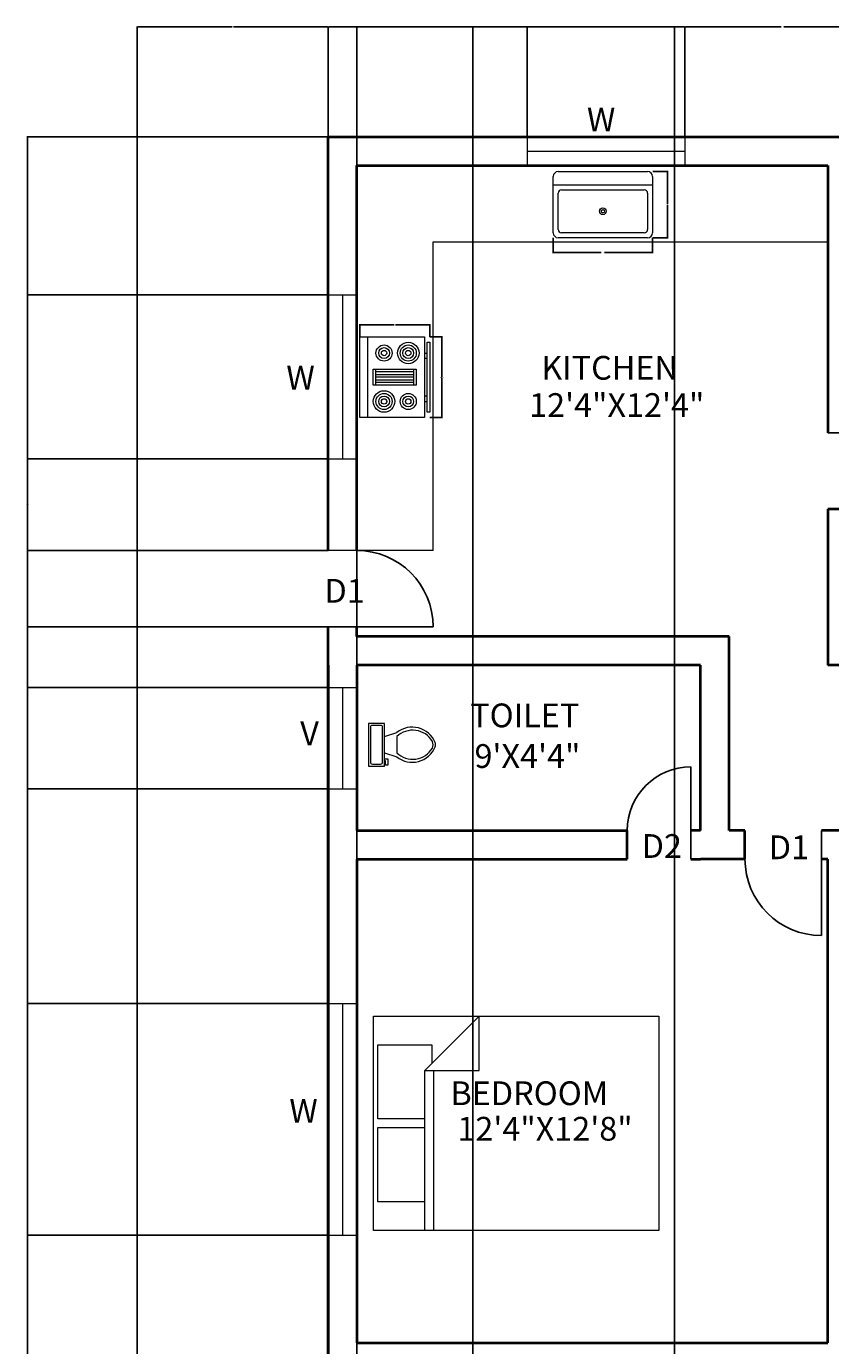
# Model space of a CAD drawing. Units: feet. Extents: x 2032 to 2763, y 1402 to 2145.
# Tile 3 of 6: x 2032 to 2285, y 1731 to 2145. Entities that reach past the tile are written whole.
import ezdxf

# ---------------------------------------------------------------- set-up
doc = ezdxf.new("R2010")
doc.units = ezdxf.units.FT
for name, color, linetype, lineweight in [('A-ANNO-DIMS', 2, 'Continuous', 18), ('A-ANNO-TEXT', 7, 'Continuous', 18), ('A-AREA-IDEN', 7, 'Continuous', 25), ('A-DOOR', 3, 'Continuous', 25), ('A-EQPM', 8, 'Continuous', 18), ('A-FLOR-CASE', 8, 'Continuous', 18), ('A-FLOR-FIXT', 8, 'Continuous', 18), ('A-FURN', 8, 'Continuous', 18), ('A-GLAZ', 4, 'Continuous', 18), ('A-WALL', 7, 'Continuous', 40), ('C-PROP', 8, 'Continuous', 25)]:
    doc.layers.add(name, color=color, linetype=linetype, lineweight=lineweight)
doc.styles.get("Standard").update_dxf_attribs({"font": 'arial.ttf'})
doc.dimstyles.get("Standard").update_dxf_attribs({"dimtxt": 0.18, "dimasz": 0.18, "dimexe": 0.18, "dimexo": 0.0625, "dimgap": 0.09, "dimtad": 0, "dimtih": 1, "dimtoh": 1, "dimdec": 4, "dimzin": 0, "dimdsep": 46, "dimtxsty": 'Standard', "dimcen": 0.09, "dimadec": 0, "dimazin": 0, "dimtfac": 1, "dimtdec": 4, "dimtofl": 0, "dimtmove": 0, "dimatfit": 3, "dimfxl": 1, "dimtolj": 1, "dimtzin": 0, "dimarcsym": 0})

# ---------------------------------------------------------------- blocks, each defined once
blk = doc.blocks.new('Sink-single - 30 in top')
blk.add_line((-15, -3.999996), (15, -3.999996))
for points in [[(-13.5, 0), (13.5, 0)], [(-15, -18.499996), (-15, -1.5)], [(15, -1.5), (15, -18.499996)], [(-13.5, -17.499996), (-13.5, -6.499996)], [(-12.5, -5.499996), (12.5, -5.499996)], [(13.5, -6.499996), (13.5, -17.499996)], [(12.5, -18.499996), (-12.5, -18.499996)], [(13.5, -19.999996), (-13.5, -19.999996)]]:
    blk.add_lwpolyline(points)
for radius in [1, 0.5]:
    blk.add_circle((0, -11.999996), radius)
for centre, radius, start, end in [((-13.5, -1.5), 1.5, 90, 180), ((13.5, -1.5), 1.5, 0, 90), ((-12.5, -6.499996), 1, 90, 180), ((12.5, -6.499996), 1, 0, 90), ((-13.5, -18.499996), 1.5, 180, 270), ((-12.5, -17.499996), 1, 180, 270), ((12.5, -17.499996), 1, 270, 0), ((13.5, -18.499996), 1.5, 270, 0)]:
    blk.add_arc(centre, radius, start, end)
blk = doc.blocks.new('Range-Oven - 30 in top')
for p, q in [((0, -3), (30, -3)), ((12, -6), (18, -6)), ((13, -20), (13, -6)), ((14, -6), (14, -20)), ((15, -20), (15, -6)), ((16, -6), (16, -20)), ((17, -20), (17, -6)), ((6, -24), (6, -25)), ((8, -25), (8, -24)), ((18, -20), (12, -20)), ((22, -25), (22, -24)), ((24, -24), (24, -25))]:
    blk.add_line(p, q)
for points in [[(0, -24), (0, 0), (30, 0), (30, -24)], [(12, -21), (12, -5), (18, -5), (18, -21)], [(2, -26), (2, -25), (28, -25), (28, -26)]]:
    blk.add_lwpolyline(points, close=True)
for centre, radius in [((6, -9), 4), ((6, -9), 3), ((6, -9), 2), ((6, -9), 1), ((24, -9), 3), ((24, -9), 2), ((24, -9), 1), ((24, -18), 4), ((6, -18), 3), ((6, -18), 2), ((6, -18), 1), ((24, -18), 3), ((24, -18), 2), ((24, -18), 1)]:
    blk.add_circle(centre, radius)
blk = doc.blocks.new('Bed - Queen')
for p, q in [((0, -80.00003), (0, 0)), ((0, 0), (59.99999, 0)), ((59.99999, 0), (59.99999, -80.00003)), ((7.99999, -1.2), (28.79998, -1.2)), ((7.99999, -14.4), (7.99999, -1.2)), ((28.79998, -1.2), (28.79998, -14.4)), ((31.19999, -1.2), (51.99999, -1.2)), ((31.19999, -14.4), (31.19999, -1.2)), ((51.99999, -1.2), (51.99999, -16.4)), ((0, -14.4), (44.8, -14.4)), ((59.99999, -29.6), (44.8, -14.4)), ((44.8, -14.4), (44.8, -29.6)), ((44.8, -16.8), (0, -16.8)), ((51.99999, -16.4), (46.79936, -16.4)), ((44.8, -29.6), (59.99999, -29.6)), ((59.99999, -80.00003), (0, -80.00003))]:
    blk.add_line(p, q)
blk = doc.blocks.new('Toilet - top')
for p, q in [((9.5, -6), (9.5, -2)), ((-10, -8.5), (-8, -8.5)), ((-10, -9.5), (-10, -8.5)), ((-7, -9.5), (-10, -9.5)), ((-8, -8.5), (-8, -8)), ((-7, -8), (-7, -9.5)), ((-4, -8), (-6, -14)), ((4, -8), (6, -14)), ((4, -14), (-4, -14))]:
    blk.add_line(p, q)
blk.add_lwpolyline([(10.5, -8), (10.5, 0), (-10.5, 0), (-10.5, -8)], close=True)
for points in [[(-9.5, -2), (-9.5, -6)], [(8.5, -1), (-8.5, -1)], [(-8.5, -7), (8.5, -7)]]:
    blk.add_lwpolyline(points)
for centre, radius, start, end in [((-8.62, -1.88), 0.884, 81.8699, 188.1301), ((-8.62, -6.12), 0.884, 171.8699, 278.1301), ((8.62, -1.88), 0.884, 351.8699, 98.1301), ((8.62, -6.12), 0.884, 261.8699, 8.1301), ((3.52, -21.58), 12.17, 141.46911, 247.97143), ((4.2, -21.82), 11.33, 136.36773, 238.94682), ((-3.52, -21.58), 12.17, 292.02843, 38.53071), ((-4.2, -21.82), 11.33, 301.05301, 43.63209), ((0, -27.88), 4, 245.73182, 294.26817), ((0, -29), 4, 254.86053, 285.13947)]:
    blk.add_arc(centre, radius, start, end)
blk = doc.blocks.new('DOOR-SWING-24')
blk.add_line((33, 0), (0, 0))
blk.add_arc((9, 0), 24, 0, 90)
blk = doc.blocks.new('DOOR-SWING-20')
blk.add_line((0, 20), (29, 20))
blk.add_arc((20, 20), 20, 180, 270)
blk = doc.blocks.new('*D27')
at = {"layer": 'A-ANNO-DIMS', "color": 0, "lineweight": -2, "transparency": 16777216}
for p, q in [((2198.05, 2078.81), (2198.05, 2074.01)), ((2229.27, 2078.81), (2229.27, 2074.01)), ((2198.23, 2074.19), (2213.13, 2074.19)), ((2229.09, 2074.19), (2214.19, 2074.19))]:
    blk.add_line(p, q, dxfattribs=at)
at = {"layer": 'A-ANNO-DIMS', "color": 0, "transparency": 16777216}
for points in [[(2198.23, 2074.22), (2198.23, 2074.16), (2198.05, 2074.19)], [(2229.09, 2074.22), (2229.09, 2074.16), (2229.27, 2074.19)]]:
    blk.add_solid(points, dxfattribs=at)
at = {"layer": 'Defpoints', "color": 0, "transparency": 16777216}
for p in [(2198.05, 2078.87), (2229.27, 2078.87), (2229.27, 2074.19)]:
    blk.add_point(p, dxfattribs=at)
at = {"layer": 'A-ANNO-DIMS', "color": 0, "transparency": 16777216, "insert": (2213.66, 2074.19), "char_height": 0.18, "attachment_point": 5}
blk.add_mtext('\\A1;SINK 31', dxfattribs=at)
blk = doc.blocks.new('*D28')
at = {"layer": 'A-ANNO-DIMS', "color": 0, "lineweight": -2, "transparency": 16777216}
for p, q in [((2229.33, 2099.68), (2234.13, 2099.68)), ((2233.95, 2099.5), (2233.95, 2089.45)), ((2233.95, 2079.05), (2233.95, 2089.09)), ((2229.33, 2078.87), (2234.13, 2078.87))]:
    blk.add_line(p, q, dxfattribs=at)
at = {"layer": 'A-ANNO-DIMS', "color": 0, "transparency": 16777216}
for points in [[(2233.92, 2099.5), (2233.98, 2099.5), (2233.95, 2099.68)], [(2233.92, 2079.05), (2233.98, 2079.05), (2233.95, 2078.87)]]:
    blk.add_solid(points, dxfattribs=at)
at = {"layer": 'Defpoints', "color": 0, "transparency": 16777216}
for p in [(2229.27, 2099.68), (2233.95, 2099.68), (2229.27, 2078.87)]:
    blk.add_point(p, dxfattribs=at)
at = {"layer": 'A-ANNO-DIMS', "color": 0, "transparency": 16777216, "insert": (2233.95, 2089.27), "char_height": 0.18, "attachment_point": 5}
blk.add_mtext('\\A1;21', dxfattribs=at)
blk = doc.blocks.new('*D29')
at = {"layer": 'A-ANNO-DIMS', "color": 0, "lineweight": -2, "transparency": 16777216}
for p, q in [((2159.3, 2047.72), (2163.22, 2047.72)), ((2163.04, 2047.54), (2163.04, 2035.22)), ((2163.04, 2022.54), (2163.04, 2034.86)), ((2159.3, 2022.36), (2163.22, 2022.36))]:
    blk.add_line(p, q, dxfattribs=at)
at = {"layer": 'A-ANNO-DIMS', "color": 0, "transparency": 16777216}
for points in [[(2163.01, 2047.54), (2163.07, 2047.54), (2163.04, 2047.72)], [(2163.01, 2022.54), (2163.07, 2022.54), (2163.04, 2022.36)]]:
    blk.add_solid(points, dxfattribs=at)
at = {"layer": 'Defpoints', "color": 0, "transparency": 16777216}
for p in [(2159.24, 2047.72), (2163.04, 2047.72), (2159.24, 2022.36)]:
    blk.add_point(p, dxfattribs=at)
at = {"layer": 'A-ANNO-DIMS', "color": 0, "transparency": 16777216, "insert": (2163.04, 2035.04), "char_height": 0.18, "attachment_point": 5}
blk.add_mtext('\\A1;RANGE 25', dxfattribs=at)
blk = doc.blocks.new('*D30')
at = {"layer": 'A-ANNO-DIMS', "color": 0, "lineweight": -2, "transparency": 16777216}
for p, q in [((2137.26, 2047.78), (2137.26, 2051.71)), ((2137.44, 2051.53), (2148.03, 2051.53)), ((2159.06, 2051.53), (2148.47, 2051.53)), ((2159.24, 2047.78), (2159.24, 2051.71))]:
    blk.add_line(p, q, dxfattribs=at)
at = {"layer": 'A-ANNO-DIMS', "color": 0, "transparency": 16777216}
for points in [[(2137.44, 2051.56), (2137.44, 2051.5), (2137.26, 2051.53)], [(2159.06, 2051.56), (2159.06, 2051.5), (2159.24, 2051.53)]]:
    blk.add_solid(points, dxfattribs=at)
at = {"layer": 'Defpoints', "color": 0, "transparency": 16777216}
for p in [(2137.26, 2051.53), (2137.26, 2047.72), (2159.24, 2047.72)]:
    blk.add_point(p, dxfattribs=at)
at = {"layer": 'A-ANNO-DIMS', "color": 0, "transparency": 16777216, "insert": (2148.25, 2051.53), "char_height": 0.18, "attachment_point": 5}
blk.add_mtext('\\A1;22', dxfattribs=at)
blk = doc.blocks.new('*D34')
at = {"layer": 'A-ANNO-DIMS', "color": 0, "lineweight": -2, "transparency": 16777216}
for p, q in [((2067.25, 2110.61), (2032.63, 2110.61)), ((2032.81, 2110.43), (2032.81, 1773.79)), ((2032.81, 1436.79), (2032.81, 1773.43)), ((2067.25, 1436.61), (2032.63, 1436.61))]:
    blk.add_line(p, q, dxfattribs=at)
at = {"layer": 'A-ANNO-DIMS', "color": 0, "transparency": 16777216}
for points in [[(2032.78, 2110.43), (2032.84, 2110.43), (2032.81, 2110.61)], [(2032.78, 1436.79), (2032.84, 1436.79), (2032.81, 1436.61)]]:
    blk.add_solid(points, dxfattribs=at)
at = {"layer": 'Defpoints', "color": 0, "transparency": 16777216}
for p in [(2032.81, 2110.61), (2067.31, 2110.61), (2067.31, 1436.61)]:
    blk.add_point(p, dxfattribs=at)
at = {"layer": 'A-ANNO-DIMS', "color": 0, "transparency": 16777216, "insert": (2032.81, 1773.61), "char_height": 0.18, "attachment_point": 5}
blk.add_mtext('\\A1;674', dxfattribs=at)
blk = doc.blocks.new('*D35')
at = {"layer": 'A-ANNO-DIMS', "color": 0, "lineweight": -2, "transparency": 16777216}
for p, q in [((2067.31, 2110.68), (2067.31, 2145.29)), ((2067.49, 2145.11), (2097.09, 2145.11)), ((2127.13, 2145.11), (2097.53, 2145.11)), ((2127.31, 2110.68), (2127.31, 2145.29))]:
    blk.add_line(p, q, dxfattribs=at)
at = {"layer": 'A-ANNO-DIMS', "color": 0, "transparency": 16777216}
for points in [[(2067.49, 2145.14), (2067.49, 2145.08), (2067.31, 2145.11)], [(2127.13, 2145.14), (2127.13, 2145.08), (2127.31, 2145.11)]]:
    blk.add_solid(points, dxfattribs=at)
at = {"layer": 'Defpoints', "color": 0, "transparency": 16777216}
for p in [(2127.31, 2145.11), (2067.31, 2110.61), (2127.31, 2110.61)]:
    blk.add_point(p, dxfattribs=at)
at = {"layer": 'A-ANNO-DIMS', "color": 0, "transparency": 16777216, "insert": (2097.31, 2145.11), "char_height": 0.18, "attachment_point": 5}
blk.add_mtext('\\A1;60', dxfattribs=at)
blk = doc.blocks.new('*D36')
at = {"layer": 'A-ANNO-DIMS', "color": 0, "lineweight": -2, "transparency": 16777216}
for p, q in [((2127.31, 2110.68), (2127.31, 2145.29)), ((2127.49, 2145.11), (2158.16, 2145.11)), ((2189.62, 2145.11), (2158.95, 2145.11)), ((2189.8, 2110.68), (2189.8, 2145.29))]:
    blk.add_line(p, q, dxfattribs=at)
at = {"layer": 'A-ANNO-DIMS', "color": 0, "transparency": 16777216}
for points in [[(2127.49, 2145.14), (2127.49, 2145.08), (2127.31, 2145.11)], [(2189.62, 2145.14), (2189.62, 2145.08), (2189.8, 2145.11)]]:
    blk.add_solid(points, dxfattribs=at)
at = {"layer": 'Defpoints', "color": 0, "transparency": 16777216}
for p in [(2189.8, 2145.11), (2127.31, 2110.61), (2189.8, 2110.61)]:
    blk.add_point(p, dxfattribs=at)
at = {"layer": 'A-ANNO-DIMS', "color": 0, "transparency": 16777216, "insert": (2158.56, 2145.11), "char_height": 0.18, "attachment_point": 5}
blk.add_mtext('\\A1;62.49', dxfattribs=at)
blk = doc.blocks.new('*D37')
at = {"layer": 'A-ANNO-DIMS', "color": 0, "lineweight": -2, "transparency": 16777216}
for p, q in [((2189.8, 2110.68), (2189.8, 2145.29)), ((2189.98, 2145.11), (2214.23, 2145.11)), ((2239.27, 2145.11), (2215.02, 2145.11)), ((2239.45, 2110.68), (2239.45, 2145.29))]:
    blk.add_line(p, q, dxfattribs=at)
at = {"layer": 'A-ANNO-DIMS', "color": 0, "transparency": 16777216}
for points in [[(2189.98, 2145.14), (2189.98, 2145.08), (2189.8, 2145.11)], [(2239.27, 2145.14), (2239.27, 2145.08), (2239.45, 2145.11)]]:
    blk.add_solid(points, dxfattribs=at)
at = {"layer": 'Defpoints', "color": 0, "transparency": 16777216}
for p in [(2239.45, 2145.11), (2189.8, 2110.61), (2239.45, 2110.61)]:
    blk.add_point(p, dxfattribs=at)
at = {"layer": 'A-ANNO-DIMS', "color": 0, "transparency": 16777216, "insert": (2214.62, 2145.11), "char_height": 0.18, "attachment_point": 5}
blk.add_mtext('\\A1;49.64', dxfattribs=at)
blk = doc.blocks.new('*D38')
at = {"layer": 'A-ANNO-DIMS', "color": 0, "lineweight": -2, "transparency": 16777216}
for p, q in [((2239.45, 2110.68), (2239.45, 2145.29)), ((2239.63, 2145.11), (2269.73, 2145.11)), ((2300.62, 2145.11), (2270.52, 2145.11)), ((2300.8, 2110.68), (2300.8, 2145.29))]:
    blk.add_line(p, q, dxfattribs=at)
at = {"layer": 'A-ANNO-DIMS', "color": 0, "transparency": 16777216}
for points in [[(2239.63, 2145.14), (2239.63, 2145.08), (2239.45, 2145.11)], [(2300.62, 2145.14), (2300.62, 2145.08), (2300.8, 2145.11)]]:
    blk.add_solid(points, dxfattribs=at)
at = {"layer": 'Defpoints', "color": 0, "transparency": 16777216}
for p in [(2300.8, 2145.11), (2239.45, 2110.61), (2300.8, 2110.61)]:
    blk.add_point(p, dxfattribs=at)
at = {"layer": 'A-ANNO-DIMS', "color": 0, "transparency": 16777216, "insert": (2270.12, 2145.11), "char_height": 0.18, "attachment_point": 5}
blk.add_mtext('\\A1;61.36', dxfattribs=at)
blk = doc.blocks.new('*D53')
at = {"layer": 'A-ANNO-DIMS', "color": 0, "lineweight": -2, "transparency": 16777216}
for p, q in [((2127.25, 1765.5), (2032.63, 1765.5)), ((2032.81, 1765.32), (2032.81, 1738.43)), ((2032.81, 1711.18), (2032.81, 1738.07)), ((2127.25, 1711), (2032.63, 1711))]:
    blk.add_line(p, q, dxfattribs=at)
at = {"layer": 'A-ANNO-DIMS', "color": 0, "transparency": 16777216}
for points in [[(2032.78, 1765.32), (2032.84, 1765.32), (2032.81, 1765.5)], [(2032.78, 1711.18), (2032.84, 1711.18), (2032.81, 1711)]]:
    blk.add_solid(points, dxfattribs=at)
at = {"layer": 'Defpoints', "color": 0, "transparency": 16777216}
for p in [(2032.81, 1765.5), (2127.31, 1765.5), (2127.31, 1711)]:
    blk.add_point(p, dxfattribs=at)
at = {"layer": 'A-ANNO-DIMS', "color": 0, "transparency": 16777216, "insert": (2032.81, 1738.25), "char_height": 0.18, "attachment_point": 5}
blk.add_mtext('\\A1;54.5', dxfattribs=at)
blk = doc.blocks.new('*D54')
at = {"layer": 'A-ANNO-DIMS', "color": 0, "lineweight": -2, "transparency": 16777216}
for p, q in [((2127.25, 1838.26), (2032.63, 1838.26)), ((2032.81, 1838.08), (2032.81, 1802.06)), ((2032.81, 1765.68), (2032.81, 1801.7)), ((2127.25, 1765.5), (2032.63, 1765.5))]:
    blk.add_line(p, q, dxfattribs=at)
at = {"layer": 'A-ANNO-DIMS', "color": 0, "transparency": 16777216}
for points in [[(2032.78, 1838.08), (2032.84, 1838.08), (2032.81, 1838.26)], [(2032.78, 1765.68), (2032.84, 1765.68), (2032.81, 1765.5)]]:
    blk.add_solid(points, dxfattribs=at)
at = {"layer": 'Defpoints', "color": 0, "transparency": 16777216}
for p in [(2032.81, 1838.26), (2127.31, 1838.26), (2127.31, 1765.5)]:
    blk.add_point(p, dxfattribs=at)
at = {"layer": 'A-ANNO-DIMS', "color": 0, "transparency": 16777216, "insert": (2032.81, 1801.88), "char_height": 0.18, "attachment_point": 5}
blk.add_mtext('\\A1;72.76', dxfattribs=at)
blk = doc.blocks.new('*D55')
at = {"layer": 'A-ANNO-DIMS', "color": 0, "lineweight": -2, "transparency": 16777216}
for p, q in [((2127.25, 1905.74), (2032.63, 1905.74)), ((2032.81, 1905.56), (2032.81, 1872.18)), ((2032.81, 1838.44), (2032.81, 1871.82)), ((2127.25, 1838.26), (2032.63, 1838.26))]:
    blk.add_line(p, q, dxfattribs=at)
at = {"layer": 'A-ANNO-DIMS', "color": 0, "transparency": 16777216}
for points in [[(2032.78, 1905.56), (2032.84, 1905.56), (2032.81, 1905.74)], [(2032.78, 1838.44), (2032.84, 1838.44), (2032.81, 1838.26)]]:
    blk.add_solid(points, dxfattribs=at)
at = {"layer": 'Defpoints', "color": 0, "transparency": 16777216}
for p in [(2032.81, 1905.74), (2127.31, 1905.74), (2127.31, 1838.26)]:
    blk.add_point(p, dxfattribs=at)
at = {"layer": 'A-ANNO-DIMS', "color": 0, "transparency": 16777216, "insert": (2032.81, 1872), "char_height": 0.18, "attachment_point": 5}
blk.add_mtext('\\A1;67.48', dxfattribs=at)
blk = doc.blocks.new('*D56')
at = {"layer": 'A-ANNO-DIMS', "color": 0, "lineweight": -2, "transparency": 16777216}
for p, q in [((2127.25, 1937.59), (2032.63, 1937.59)), ((2032.81, 1937.41), (2032.81, 1921.85)), ((2032.81, 1905.92), (2032.81, 1921.48)), ((2127.25, 1905.74), (2032.63, 1905.74))]:
    blk.add_line(p, q, dxfattribs=at)
at = {"layer": 'A-ANNO-DIMS', "color": 0, "transparency": 16777216}
for points in [[(2032.78, 1937.41), (2032.84, 1937.41), (2032.81, 1937.59)], [(2032.78, 1905.92), (2032.84, 1905.92), (2032.81, 1905.74)]]:
    blk.add_solid(points, dxfattribs=at)
at = {"layer": 'Defpoints', "color": 0, "transparency": 16777216}
for p in [(2032.81, 1937.59), (2127.31, 1937.59), (2127.31, 1905.74)]:
    blk.add_point(p, dxfattribs=at)
at = {"layer": 'A-ANNO-DIMS', "color": 0, "transparency": 16777216, "insert": (2032.81, 1921.66), "char_height": 0.18, "attachment_point": 5}
blk.add_mtext('\\A1;31.85', dxfattribs=at)
blk = doc.blocks.new('*D57')
at = {"layer": 'A-ANNO-DIMS', "color": 0, "lineweight": -2, "transparency": 16777216}
for p, q in [((2127.25, 1956.61), (2032.63, 1956.61)), ((2032.81, 1956.43), (2032.81, 1947.28)), ((2032.81, 1937.77), (2032.81, 1946.92)), ((2127.25, 1937.59), (2032.63, 1937.59))]:
    blk.add_line(p, q, dxfattribs=at)
at = {"layer": 'A-ANNO-DIMS', "color": 0, "transparency": 16777216}
for points in [[(2032.78, 1956.43), (2032.84, 1956.43), (2032.81, 1956.61)], [(2032.78, 1937.77), (2032.84, 1937.77), (2032.81, 1937.59)]]:
    blk.add_solid(points, dxfattribs=at)
at = {"layer": 'Defpoints', "color": 0, "transparency": 16777216}
for p in [(2032.81, 1956.61), (2127.31, 1956.61), (2127.31, 1937.59)]:
    blk.add_point(p, dxfattribs=at)
at = {"layer": 'A-ANNO-DIMS', "color": 0, "transparency": 16777216, "insert": (2032.81, 1947.1), "char_height": 0.18, "attachment_point": 5}
blk.add_mtext('\\A1;19.025', dxfattribs=at)
blk = doc.blocks.new('*D58')
at = {"layer": 'A-ANNO-DIMS', "color": 0, "lineweight": -2, "transparency": 16777216}
for p, q in [((2127.25, 1980.61), (2032.63, 1980.61)), ((2032.81, 1980.43), (2032.81, 1968.79)), ((2032.81, 1956.79), (2032.81, 1968.43)), ((2127.25, 1956.61), (2032.63, 1956.61))]:
    blk.add_line(p, q, dxfattribs=at)
at = {"layer": 'A-ANNO-DIMS', "color": 0, "transparency": 16777216}
for points in [[(2032.78, 1980.43), (2032.84, 1980.43), (2032.81, 1980.61)], [(2032.78, 1956.79), (2032.84, 1956.79), (2032.81, 1956.61)]]:
    blk.add_solid(points, dxfattribs=at)
at = {"layer": 'Defpoints', "color": 0, "transparency": 16777216}
for p in [(2032.81, 1980.61), (2127.31, 1980.61), (2127.31, 1956.61)]:
    blk.add_point(p, dxfattribs=at)
at = {"layer": 'A-ANNO-DIMS', "color": 0, "transparency": 16777216, "insert": (2032.81, 1968.61), "char_height": 0.18, "attachment_point": 5}
blk.add_mtext('\\A1;24', dxfattribs=at)
blk = doc.blocks.new('*D59')
at = {"layer": 'A-ANNO-DIMS', "color": 0, "lineweight": -2, "transparency": 16777216}
for p, q in [((2127.25, 2009.42), (2032.63, 2009.42)), ((2032.81, 2009.24), (2032.81, 1995.2)), ((2032.81, 1980.79), (2032.81, 1994.83)), ((2127.25, 1980.61), (2032.63, 1980.61))]:
    blk.add_line(p, q, dxfattribs=at)
at = {"layer": 'A-ANNO-DIMS', "color": 0, "transparency": 16777216}
for points in [[(2032.78, 2009.24), (2032.84, 2009.24), (2032.81, 2009.42)], [(2032.78, 1980.79), (2032.84, 1980.79), (2032.81, 1980.61)]]:
    blk.add_solid(points, dxfattribs=at)
at = {"layer": 'Defpoints', "color": 0, "transparency": 16777216}
for p in [(2032.81, 2009.42), (2127.31, 2009.42), (2127.31, 1980.61)]:
    blk.add_point(p, dxfattribs=at)
at = {"layer": 'A-ANNO-DIMS', "color": 0, "transparency": 16777216, "insert": (2032.81, 1995.02), "char_height": 0.18, "attachment_point": 5}
blk.add_mtext('\\A1;28.807', dxfattribs=at)
blk = doc.blocks.new('*D60')
at = {"layer": 'A-ANNO-DIMS', "color": 0, "lineweight": -2, "transparency": 16777216}
for p, q in [((2127.25, 2060.94), (2032.63, 2060.94)), ((2032.81, 2060.76), (2032.81, 2035.36)), ((2032.81, 2009.6), (2032.81, 2035)), ((2127.25, 2009.42), (2032.63, 2009.42))]:
    blk.add_line(p, q, dxfattribs=at)
at = {"layer": 'A-ANNO-DIMS', "color": 0, "transparency": 16777216}
for points in [[(2032.78, 2060.76), (2032.84, 2060.76), (2032.81, 2060.94)], [(2032.78, 2009.6), (2032.84, 2009.6), (2032.81, 2009.42)]]:
    blk.add_solid(points, dxfattribs=at)
at = {"layer": 'Defpoints', "color": 0, "transparency": 16777216}
for p in [(2032.81, 2060.94), (2127.31, 2060.94), (2127.31, 2009.42)]:
    blk.add_point(p, dxfattribs=at)
at = {"layer": 'A-ANNO-DIMS', "color": 0, "transparency": 16777216, "insert": (2032.81, 2035.18), "char_height": 0.18, "attachment_point": 5}
blk.add_mtext('\\A1;51.52', dxfattribs=at)
blk = doc.blocks.new('*D61')
at = {"layer": 'A-ANNO-DIMS', "color": 0, "lineweight": -2, "transparency": 16777216}
for p, q in [((2127.25, 2110.61), (2032.63, 2110.61)), ((2032.81, 2110.43), (2032.81, 2085.96)), ((2032.81, 2061.12), (2032.81, 2085.59)), ((2127.25, 2060.94), (2032.63, 2060.94))]:
    blk.add_line(p, q, dxfattribs=at)
at = {"layer": 'A-ANNO-DIMS', "color": 0, "transparency": 16777216}
for points in [[(2032.78, 2110.43), (2032.84, 2110.43), (2032.81, 2110.61)], [(2032.78, 2061.12), (2032.84, 2061.12), (2032.81, 2060.94)]]:
    blk.add_solid(points, dxfattribs=at)
at = {"layer": 'Defpoints', "color": 0, "transparency": 16777216}
for p in [(2032.81, 2110.61), (2127.31, 2110.61), (2127.31, 2060.94)]:
    blk.add_point(p, dxfattribs=at)
at = {"layer": 'A-ANNO-DIMS', "color": 0, "transparency": 16777216, "insert": (2032.81, 2085.78), "char_height": 0.18, "attachment_point": 5}
blk.add_mtext('\\A1;49.68', dxfattribs=at)
blk = doc.blocks.new('*D70')
at = {"layer": 'A-ANNO-DIMS', "color": 0, "lineweight": -2, "transparency": 16777216}
for p, q in [((2136.31, 1505.68), (2136.31, 2145.29)), ((2136.49, 2145.11), (2154.19, 2145.11)), ((2172.54, 2145.11), (2154.84, 2145.11)), ((2172.72, 1505.68), (2172.72, 2145.29))]:
    blk.add_line(p, q, dxfattribs=at)
at = {"layer": 'A-ANNO-DIMS', "color": 0, "transparency": 16777216}
for points in [[(2136.49, 2145.14), (2136.49, 2145.08), (2136.31, 2145.11)], [(2172.54, 2145.14), (2172.54, 2145.08), (2172.72, 2145.11)]]:
    blk.add_solid(points, dxfattribs=at)
at = {"layer": 'Defpoints', "color": 0, "transparency": 16777216}
for p in [(2172.72, 2145.11), (2136.31, 1505.61), (2172.72, 1505.61)]:
    blk.add_point(p, dxfattribs=at)
at = {"layer": 'A-ANNO-DIMS', "color": 0, "transparency": 16777216, "insert": (2154.51, 2145.11), "char_height": 0.18, "attachment_point": 5}
blk.add_mtext('\\A1;36.4', dxfattribs=at)
blk = doc.blocks.new('*D71')
at = {"layer": 'A-ANNO-DIMS', "color": 0, "lineweight": -2, "transparency": 16777216}
for p, q in [((2172.72, 1505.68), (2172.72, 2145.29)), ((2172.9, 2145.11), (2204.05, 2145.11)), ((2236, 2145.11), (2204.84, 2145.11)), ((2236.18, 1505.68), (2236.18, 2145.29))]:
    blk.add_line(p, q, dxfattribs=at)
at = {"layer": 'A-ANNO-DIMS', "color": 0, "transparency": 16777216}
for points in [[(2172.9, 2145.14), (2172.9, 2145.08), (2172.72, 2145.11)], [(2236, 2145.14), (2236, 2145.08), (2236.18, 2145.11)]]:
    blk.add_solid(points, dxfattribs=at)
at = {"layer": 'Defpoints', "color": 0, "transparency": 16777216}
for p in [(2236.18, 2145.11), (2172.72, 1505.61), (2236.18, 1505.61)]:
    blk.add_point(p, dxfattribs=at)
at = {"layer": 'A-ANNO-DIMS', "color": 0, "transparency": 16777216, "insert": (2204.45, 2145.11), "char_height": 0.18, "attachment_point": 5}
blk.add_mtext('\\A1;63.46', dxfattribs=at)

msp = doc.modelspace()

# ---------------------------------------------------------------- linework, layer by layer
at = {"layer": 'A-FLOR-CASE'}
for p, q in [((2160.3136, 2077.6131), (2284.3136, 2077.6131)), ((2160.3136, 1980.6131), (2160.3136, 2077.6131)), ((2160.3136, 1980.6131), (2127.3136, 1980.6131))]:
    msp.add_line(p, q, dxfattribs=at)
at = {"layer": 'A-GLAZ'}
for p, q in [((2189.8034, 2110.6131), (2189.8034, 2101.6131)), ((2239.4453, 2110.6131), (2239.4453, 2101.6131)), ((2189.8034, 2106.1131), (2239.4453, 2106.1131)), ((2127.3136, 2060.9373), (2136.3136, 2060.9373)), ((2131.8136, 2060.9373), (2131.8136, 2009.42)), ((2127.3136, 2009.42), (2136.3136, 2009.42)), ((2127.3136, 1937.5885), (2136.3136, 1937.5885)), ((2131.8136, 1937.5885), (2131.8136, 1905.7409)), ((2127.3136, 1905.7409), (2136.3136, 1905.7409)), ((2127.3136, 1838.2613), (2136.3136, 1838.2613)), ((2131.8136, 1838.2613), (2131.8136, 1765.4989)), ((2127.3136, 1765.4989), (2136.3136, 1765.4989))]:
    msp.add_line(p, q, dxfattribs=at)
at = {"layer": 'A-WALL'}
for p, q in [((2127.3136, 2110.6131), (2284.3136, 2110.6131)), ((2127.3136, 2110.6131), (2515.3136, 2110.6131)), ((2127.3136, 2110.6131), (2515.3136, 2110.6131)), ((2127.3136, 1980.6131), (2127.3136, 2110.6131)), ((2136.3136, 2101.6131), (2284.3136, 2101.6131)), ((2136.3136, 1980.6131), (2136.3136, 2101.6131)), ((2284.3136, 2101.6131), (2284.3136, 2017.6131)), ((2293.3136, 1993.6131), (2284.3136, 1993.6131)), ((2284.3136, 1993.6131), (2284.3136, 1944.6131)), ((2127.3136, 1496.6131), (2127.3136, 1956.6131)), ((2136.3136, 1953.6131), (2136.3136, 1956.6131)), ((2253.3136, 1953.6131), (2136.3136, 1953.6131)), ((2253.3136, 1892.6131), (2253.3136, 1953.6131)), ((2127.3136, 1944.6131), (2127.3136, 1496.6131)), ((2136.3136, 1944.6131), (2136.3136, 1892.6131)), ((2244.3136, 1944.6131), (2136.3136, 1944.6131)), ((2244.3136, 1892.6131), (2244.3136, 1944.6131)), ((2494.3136, 1944.6131), (2284.3136, 1944.6131)), ((2136.3136, 1892.6131), (2221.3136, 1892.6131)), ((2221.3136, 1883.6131), (2221.3136, 1892.6131)), ((2244.3136, 1892.6131), (2241.3136, 1892.6131)), ((2258.3136, 1892.6131), (2253.3136, 1892.6131)), ((2258.3136, 1883.6131), (2258.3136, 1892.6131)), ((2293.3136, 1892.6131), (2282.3136, 1892.6131)), ((2127.3136, 1883.6131), (2127.3136, 1731.6131)), ((2136.3136, 1883.6131), (2221.3136, 1883.6131)), ((2136.3136, 1883.6131), (2136.3136, 1731.6131)), ((2241.3136, 1883.6131), (2244.3136, 1883.6131)), ((2258.3136, 1883.6131), (2244.3136, 1883.6131)), ((2284.3136, 1883.6131), (2282.3136, 1883.6131)), ((2284.3136, 1731.6131), (2284.3136, 1883.6131)), ((2136.3136, 1731.6131), (2284.3136, 1731.6131))]:
    msp.add_line(p, q, dxfattribs=at)
at = {"layer": 'C-PROP'}
for p, q in [((2127.3136, 2110.6131), (2067.3136, 2110.6131)), ((2067.3136, 2110.6131), (2067.3136, 1436.6131))]:
    msp.add_line(p, q, dxfattribs=at)

# ---------------------------------------------------------------- block references
at = {"layer": 'A-DOOR', "extrusion": (0, 0, -1), "zscale": -1}
for p, rotation in [((-2284.314, 2017.6131), 180), ((-2282.3137, 1892.6127), 269.9999999999988)]:
    msp.add_blockref('DOOR-SWING-24', p, dxfattribs=dict(at, rotation=rotation))
at = {"layer": 'A-DOOR'}
msp.add_blockref('DOOR-SWING-24', (2127.314, 1956.613), dxfattribs=at)
at = {"layer": 'A-DOOR', "rotation": 270}
msp.add_blockref('DOOR-SWING-20', (2221.3136, 1912.6127), dxfattribs=at)
at = {"layer": 'A-EQPM', "xscale": 0.8453592349900645, "yscale": 0.8453592349900645, "zscale": 0.8453592349900645, "rotation": 90}
msp.add_blockref('Range-Oven - 30 in top', (2137.2578, 2022.3602), dxfattribs=at)
at = {"layer": 'A-FLOR-FIXT', "xscale": 1.04056653052336, "yscale": 1.04056653052336, "zscale": 1.04056653052336}
msp.add_blockref('Sink-single - 30 in top', (2213.6616, 2099.6798), dxfattribs=at)
at = {"layer": 'A-FLOR-FIXT', "xscale": 0.6388725113463674, "yscale": 0.6388725113463674, "zscale": 0.6388725113463674, "rotation": 90}
msp.add_blockref('Toilet - top', (2139.9337, 1919.5774), dxfattribs=at)
at = {"layer": 'A-FURN', "xscale": 1.121589901058193, "yscale": 1.121589901058193, "zscale": 1.121589901058193, "rotation": 90}
msp.add_blockref('Bed - Queen', (2141.5258, 1766.9746), dxfattribs=at)

# ---------------------------------------------------------------- texts
at = {"layer": 'A-ANNO-TEXT'}
for s, height, p in [('W', 7.4682, (2208.6287, 2112.329)), ('W', 7.4682, (2114.1497, 2031.1811)), ('D1', 7.46821, (2126.145, 1964.2018)), ('V', 7.4682, (2118.5085, 1919.4286)), ('D2', 7.46821, (2225.8265, 1884.0023)), ('D1', 7.46821, (2265.785, 1883.6085)), ('W', 7.4682, (2115.0798, 1800.8105))]:
    msp.add_text(s, height=height, dxfattribs=at).set_placement(p)
at = {"layer": 'A-AREA-IDEN'}
for s, height, p in [('KITCHEN', 7.46821, (2194.287, 2034.2679)), ('12\'4"X12\'4"', 7.468214, (2190.4588, 2022.5673)), ('TOILET', 7.46821, (2171.9498, 1925.0562)), ('9\'X4\'4"', 7.46821, (2173.2883, 1912.2871)), ('BEDROOM', 7.46821, (2165.7319, 1806.3266)), ('12\'4"X12\'8"', 7.468214, (2167.9087, 1795.1654))]:
    msp.add_text(s, height=height, dxfattribs=at).set_placement(p)

# ---------------------------------------------------------------- dimensions: what is measured, and where the dimension line sits
at = {"layer": 'A-ANNO-DIMS'}
for base, p1, p2, override, picture, middle in [((2127.3136, 2145.1131), (2067.3136, 2110.6131), (2127.3136, 2110.6131), {"dimdec": 0, "dimlfac": 1, "dimrnd": 0, "dimzin": 0, "dimdsep": 46, "dimlunit": 2}, '*D35', (2097.3136, 2145.1131)), ((2189.8034, 2145.1131), (2127.3136, 2110.6131), (2189.8034, 2110.6131), {"dimdec": 2, "dimlfac": 1, "dimrnd": 0, "dimzin": 0, "dimdsep": 46, "dimlunit": 2}, '*D36', (2158.5585, 2145.1131)), ((2172.7162, 2145.1131), (2136.3136, 1505.6131), (2172.7162, 1505.6131), {"dimdec": 1, "dimlfac": 1, "dimrnd": 0, "dimzin": 0, "dimdsep": 46, "dimlunit": 2}, '*D70', (2154.5149, 2145.1131)), ((2236.1806, 2145.1131), (2172.7162, 1505.6131), (2236.1806, 1505.6131), {"dimdec": 2, "dimlfac": 1, "dimrnd": 0, "dimzin": 0, "dimdsep": 46, "dimlunit": 2}, '*D71', (2204.4484, 2145.1131)), ((2239.4453, 2145.1131), (2189.8034, 2110.6131), (2239.4453, 2110.6131), {"dimdec": 2, "dimlfac": 1, "dimrnd": 0, "dimzin": 0, "dimdsep": 46, "dimlunit": 2}, '*D37', (2214.6244, 2145.1131)), ((2300.80031, 2145.11307), (2239.44528, 2110.61307), (2300.80031, 2110.61307), {"dimdec": 2, "dimlfac": 1, "dimrnd": 0, "dimzin": 0, "dimdsep": 46, "dimlunit": 2}, '*D38', (2270.12279, 2145.11307))]:
    dim = msp.add_linear_dim(base=base, p1=p1, p2=p2, dimstyle='Standard', override=override, dxfattribs=at)
    dim.commit()
    dim.dimension.update_dxf_attribs({"geometry": picture, "text_midpoint": middle})
for base, p1, p2, angle, override, picture, middle in [((2032.8136, 2110.6131), (2127.3136, 2060.9373), (2127.3136, 2110.6131), 90, {"dimdec": 2, "dimlfac": 1, "dimrnd": 0, "dimzin": 0, "dimdsep": 46, "dimlunit": 2}, '*D61', (2032.8136, 2085.7752)), ((2032.8136, 2110.6131), (2067.3136, 1436.6131), (2067.3136, 2110.6131), 90, {"dimdec": 0, "dimlfac": 1, "dimrnd": 0, "dimzin": 0, "dimdsep": 46, "dimlunit": 2}, '*D34', (2032.8136, 1773.6131)), ((2233.9526, 2099.6798), (2229.2701, 2078.8684), (2229.2701, 2099.6798), 90, {"dimdec": 0, "dimlfac": 1, "dimrnd": 0, "dimzin": 0, "dimdsep": 46, "dimlunit": 2}, '*D28', (2233.9526, 2089.2741)), ((2032.8136, 2060.9373), (2127.3136, 2009.42), (2127.3136, 2060.9373), 90, {"dimdec": 2, "dimlfac": 1, "dimrnd": 0, "dimzin": 0, "dimdsep": 46, "dimlunit": 2}, '*D60', (2032.8136, 2035.1786)), ((2137.2578, 2051.5251), (2159.2371, 2047.721), (2137.2578, 2047.721), 180, {"dimdec": 0, "dimlfac": 1, "dimrnd": 0, "dimzin": 0, "dimdsep": 46, "dimlunit": 2}, '*D30', (2148.2474, 2051.5251)), ((2032.8136, 2009.42), (2127.3136, 1980.6131), (2127.3136, 2009.42), 90, {"dimdec": 3, "dimlfac": 1, "dimrnd": 0, "dimzin": 0, "dimdsep": 46, "dimlunit": 2}, '*D59', (2032.8136, 1995.0165)), ((2032.8136, 1980.6131), (2127.3136, 1956.6131), (2127.3136, 1980.6131), 90, {"dimdec": 0, "dimlfac": 1, "dimrnd": 0, "dimzin": 0, "dimdsep": 46, "dimlunit": 2}, '*D58', (2032.8136, 1968.6131)), ((2032.8136, 1956.6131), (2127.3136, 1937.5885), (2127.3136, 1956.6131), 90, {"dimdec": 3, "dimlfac": 1, "dimrnd": 0, "dimzin": 0, "dimdsep": 46, "dimlunit": 2}, '*D57', (2032.8136, 1947.1008)), ((2032.8136, 1937.5885), (2127.3136, 1905.7409), (2127.3136, 1937.5885), 90, {"dimdec": 2, "dimlfac": 1, "dimrnd": 0, "dimzin": 0, "dimdsep": 46, "dimlunit": 2}, '*D56', (2032.8136, 1921.6647)), ((2032.8136, 1905.7409), (2127.3136, 1838.2613), (2127.3136, 1905.7409), 90, {"dimdec": 2, "dimlfac": 1, "dimrnd": 0, "dimzin": 0, "dimdsep": 46, "dimlunit": 2}, '*D55', (2032.8136, 1872.0011)), ((2032.8136, 1838.2613), (2127.3136, 1765.4989), (2127.3136, 1838.2613), 90, {"dimdec": 2, "dimlfac": 1, "dimrnd": 0, "dimzin": 0, "dimdsep": 46, "dimlunit": 2}, '*D54', (2032.8136, 1801.8801)), ((2032.8136, 1765.4989), (2127.3136, 1710.9972), (2127.3136, 1765.4989), 90, {"dimdec": 1, "dimlfac": 1, "dimrnd": 0, "dimzin": 0, "dimdsep": 46, "dimlunit": 2}, '*D53', (2032.8136, 1738.2481))]:
    dim = msp.add_linear_dim(base=base, p1=p1, p2=p2, angle=angle, dimstyle='Standard', override=override, dxfattribs=at)
    dim.commit()
    dim.dimension.update_dxf_attribs({"geometry": picture, "text_midpoint": middle})
dim = msp.add_linear_dim(base=(2229.2701, 2074.1859), p1=(2198.0531, 2078.8684), p2=(2229.2701, 2078.8684), text='SINK <>', dimstyle='Standard', override={"dimdec": 0, "dimlfac": 1, "dimrnd": 0, "dimzin": 0, "dimdsep": 46, "dimlunit": 2}, dxfattribs=at)
dim.commit()
dim.dimension.update_dxf_attribs({"geometry": '*D27', "text_midpoint": (2213.6616, 2074.1859)})
dim = msp.add_linear_dim(base=(2163.0412, 2047.721), p1=(2159.2371, 2022.3602), p2=(2159.2371, 2047.721), angle=90, text='RANGE <>', dimstyle='Standard', override={"dimdec": 0, "dimlfac": 1, "dimrnd": 0, "dimzin": 0, "dimdsep": 46, "dimlunit": 2}, dxfattribs=at)
dim.commit()
dim.dimension.update_dxf_attribs({"geometry": '*D29', "text_midpoint": (2163.0412, 2035.0406)})

doc.saveas('drawing.dxf')
